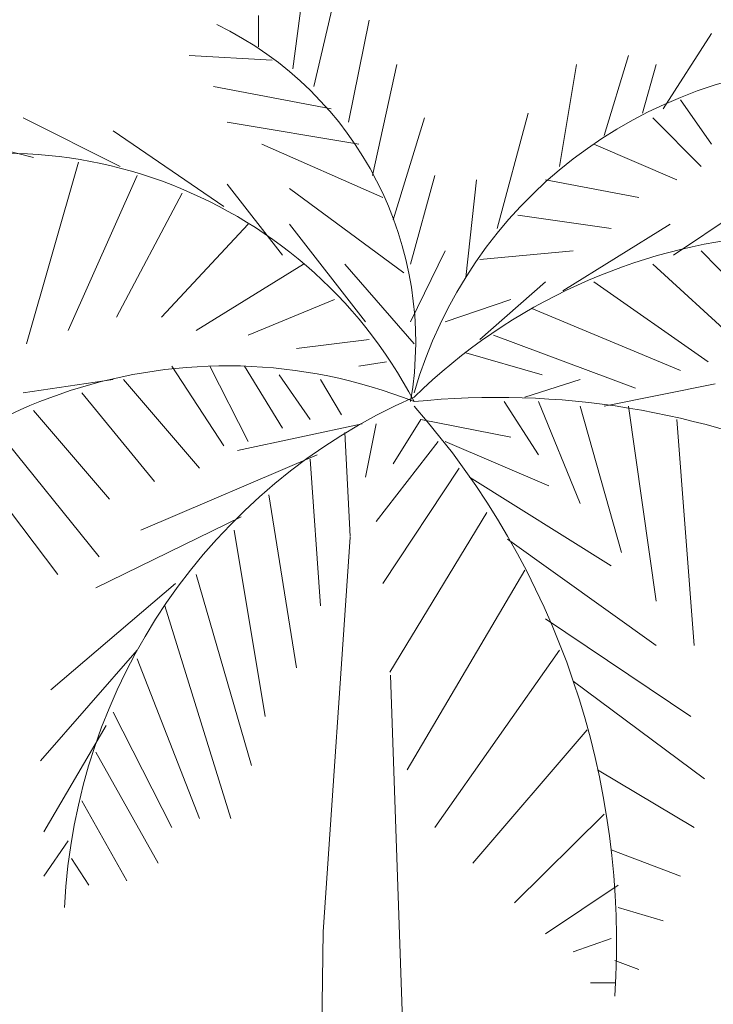
# Model space of a CAD drawing. Units: inches. Extents: x 37 to 824, y -700 to 234.
# Tile 5 of 77: x 110 to 149, y -459 to -404. Entities that reach past the tile are written whole.
import ezdxf

# ---------------------------------------------------------------- set-up
doc = ezdxf.new("R2010")
doc.units = ezdxf.units.IN
doc.header["$MEASUREMENT"] = 0
doc.layers.add('A-SITE-PLNT', color=3, linetype='Continuous', lineweight=13)

# ---------------------------------------------------------------- blocks, each defined once
blk = doc.blocks.new('*U34')
for p, q in [((-5.567, 196.707), (-4.987, 201.167)), ((-4.407, 195.716), (-3.247, 200.672)), ((-7.5, 199.68), (-7.5, 197.946)), ((-2.474, 193.733), (-1.315, 199.433)), ((15.116, 194.477), (17.822, 198.689)), ((-6.727, 197.202), (-11.366, 197.45)), ((11.829, 192.99), (13.182, 197.45)), ((-1.121, 190.759), (0.232, 196.955)), ((9.317, 191.255), (10.283, 196.955)), ((13.956, 194.229), (14.729, 196.955)), ((-3.441, 194.477), (-10.013, 195.716)), ((16.082, 194.972), (17.822, 192.494)), ((5.837, 187.786), (7.577, 194.229)), ((-15.232, 191.255), (-20.644, 193.981)), ((-1.894, 192.494), (-9.24, 193.733)), ((0.038, 188.281), (1.778, 193.981)), ((14.536, 193.981), (17.242, 191.255)), ((-20.064, 191.751), (-25.863, 193.238)), ((-9.433, 189.025), (-15.618, 193.238)), ((-0.541, 189.52), (-7.307, 192.494)), ((11.25, 192.494), (15.889, 190.512)), ((-17.551, 191.503), (-20.451, 181.343)), ((-14.265, 190.759), (-18.131, 182.086)), ((1.005, 185.803), (2.358, 190.759)), ((4.098, 185.06), (4.678, 190.512)), ((8.544, 190.512), (13.763, 189.52)), ((-11.753, 189.768), (-15.425, 182.83)), ((-6.147, 186.299), (-9.24, 190.264)), ((-5.76, 190.016), (0.618, 185.308)), ((15.695, 186.299), (19.368, 188.777)), ((6.997, 188.529), (12.216, 187.786)), ((-8.08, 188.034), (-12.912, 182.83)), ((-5.76, 188.034), (-1.508, 182.582)), ((9.51, 184.317), (15.502, 188.034)), ((1.005, 182.582), (2.938, 186.547)), ((4.871, 186.051), (10.09, 186.547)), ((17.242, 186.547), (23.041, 180.599)), ((-4.987, 185.803), (-10.979, 182.086)), ((-2.668, 185.803), (1.198, 181.343)), ((14.536, 185.803), (19.948, 180.847)), ((4.871, 181.591), (8.544, 184.812)), ((11.25, 184.812), (17.628, 180.352)), ((-3.247, 183.821), (-8.08, 181.838)), ((2.938, 182.582), (6.61, 183.821)), ((7.77, 183.325), (16.082, 179.856)), ((-1.315, 181.591), (-5.374, 181.095)), ((5.644, 181.838), (13.569, 178.865)), ((4.098, 180.847), (8.35, 179.608)), ((-12.332, 180.104), (-9.433, 175.643)), ((-10.206, 180.104), (-8.08, 175.891)), ((-8.273, 180.104), (-6.147, 176.635)), ((-0.348, 180.352), (-1.894, 180.104)), ((-15.618, 179.36), (-20.644, 178.617)), ((-15.038, 179.36), (-10.786, 174.404)), ((-6.34, 179.608), (-4.6, 177.13)), ((-4.021, 179.36), (-2.861, 177.378)), ((7.384, 178.369), (10.476, 179.36)), ((11.829, 177.874), (18.015, 179.113)), ((-17.358, 178.617), (-13.299, 173.661)), ((6.224, 178.121), (8.157, 175.148)), ((8.157, 178.121), (10.476, 172.422)), ((10.476, 177.874), (12.796, 169.696)), ((13.182, 177.874), (14.729, 166.97)), ((-20.064, 177.626), (-15.812, 172.67)), ((1.585, 177.13), (0.038, 174.652)), ((1.585, 177.13), (6.61, 176.139)), ((15.889, 177.13), (16.855, 164.492)), ((-22.191, 176.635), (-16.391, 169.448)), ((-1.701, 176.882), (-8.66, 175.396)), ((-0.928, 176.882), (-1.508, 173.909)), ((-2.668, 176.387), (-2.376, 170.594)), ((-24.317, 175.891), (-18.711, 168.457)), ((2.551, 175.891), (-0.928, 171.431)), ((2.938, 175.891), (8.737, 173.413)), ((-4.214, 175.148), (-14.072, 170.935)), ((-4.6, 174.9), (-4.021, 166.722)), ((3.711, 174.404), (-0.541, 167.961)), ((4.291, 173.909), (12.216, 168.953)), ((-6.92, 172.917), (-5.374, 163.253)), ((-8.466, 171.678), (-16.585, 167.713)), ((5.257, 171.926), (-0.155, 163.005)), ((-8.853, 170.935), (-7.113, 160.527)), ((6.417, 170.439), (14.729, 164.492)), ((-10.979, 168.457), (-7.887, 157.801)), ((7.384, 168.705), (0.812, 157.553)), ((-12.139, 167.961), (-19.098, 162.014)), ((-12.719, 166.722), (-9.046, 154.828)), ((8.544, 165.979), (16.662, 160.527)), ((-14.265, 164.244), (-19.678, 158.049)), ((9.317, 164.244), (2.358, 154.332)), ((-14.265, 163.749), (-10.786, 154.828)), ((10.09, 162.51), (17.435, 157.058)), ((-15.618, 160.775), (-12.332, 154.332)), ((-16.005, 160.031), (-19.484, 154.084)), ((10.863, 159.784), (4.484, 152.35)), ((-16.585, 158.545), (-13.106, 152.35)), ((11.443, 157.553), (16.855, 154.332)), ((-17.358, 155.819), (-14.845, 151.358)), ((11.829, 155.075), (6.804, 150.119)), ((-18.131, 153.589), (-19.484, 151.606)), ((12.216, 153.093), (16.082, 151.606)), ((-17.938, 152.597), (-16.972, 151.111)), ((12.603, 151.111), (8.544, 148.385)), ((12.603, 149.872), (15.116, 149.128)), ((12.216, 148.137), (10.09, 147.393)), ((12.409, 146.898), (13.763, 146.402)), ((12.409, 145.659), (11.056, 145.659))]:
    blk.add_line(p, q)
for points in [[(-2.363, 170.553), (-3.88, 148.505), (-4.988, 69.634), (-3.325, 24.869), (0, 0)], [(-0.116, 162.848), (0.554, 143.532), (2.217, 96.635), (3.88, 44.054), (7.76, 12.079), (11.64, 0)]]:
    blk.add_lwpolyline(points)
for centre, radius, start, end in [((-18.427, 181.448), 19.715, 350.285, 64.1123), ((25.595, 171.567), 25.395, 91.4032, 163.882), ((-21.738, 166.094), 25.899, 27.6712, 112.5305), ((23.687, 155.341), 32.188, 56.1927, 134.3213), ((-9.259, 151.732), 28.386, 68.3831, 147.5322), ((14.394, 148.393), 32.752, 113.7592, 177.4133), ((5.828, 132.718), 45.639, 35.9878, 95.8227), ((-32.8, 147.923), 45.309, 356.1943, 41.3785)]:
    blk.add_arc(centre, radius, start, end)

msp = doc.modelspace()

# ---------------------------------------------------------------- block references
at = {"layer": 'A-SITE-PLNT'}
msp.add_blockref('*U34', (131.077, -603.627), dxfattribs=at)

doc.saveas('drawing.dxf')
